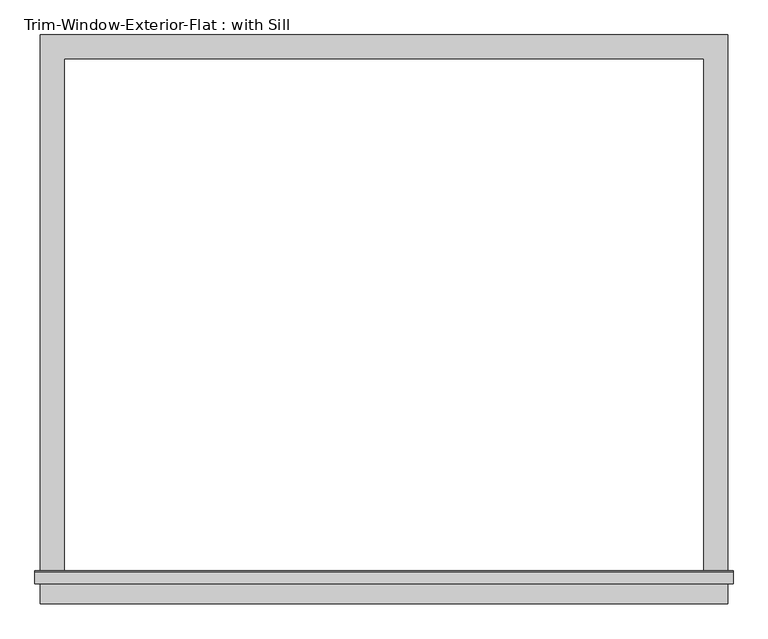
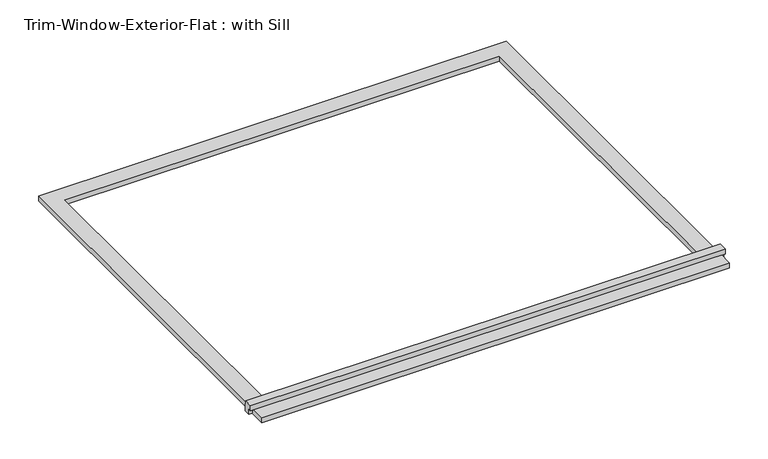
"""IFC4 building model written with IfcOpenShell, lengths in millimetres: proxy geometry, Trim-Window-Exterior-Flat : with Sill."""

from ifc_helpers import new_model, si_unit, frame, origin, origin_with_axes, place, context, project, spatial, polyline, outline, extrude, source, transform, mapped, element, save


def trim_window_exterior_flat_with_sill_7631c5ba(model_context):
    return source(origin(), model_context, "Body", "SweptSolid", [
        extrude(outline(polyline([(819.15, -1241.3823709), (819.15, -1298.5323709), (-819.15, -1298.5323709), (-819.15, -1241.3823709), (819.15, -1241.3823709)])), origin_with_axes(), (0.0, 0.0, 1.0), 19.05),
        extrude(outline(polyline([(-1250.95, 38.1), (-1221.6580645, 38.1), (-1219.2, 19.05), (-1219.2, 0.0), (-1241.3823709, 0.0), (-1241.3823709, 19.05), (-1250.95, 19.05), (-1250.95, 38.1)])), frame((-831.85, 0.0, 0.0), z_axis=(1.0, 0.0, 0.0), x_axis=(0.0, 1.0, 0.0)), (0.0, 0.0, 1.0), 1663.7),
        extrude(outline(polyline([(-819.15, 57.15), (819.15, 57.15), (819.15, -1219.2), (762.0, -1219.2), (762.0, 0.0), (-762.0, 0.0), (-762.0, -1219.2), (-819.15, -1219.2), (-819.15, 57.15)])), origin_with_axes(), (0.0, 0.0, 1.0), 19.05),
    ])


if __name__ == "__main__":
    model = new_model("IFC4")
    model_context = context("Model", 3, world=origin())
    ifc_project = project(units=[si_unit("LENGTHUNIT", "METRE", prefix="MILLI")], contexts=[model_context])
    site = spatial("IfcSite", under=ifc_project)
    building = spatial("IfcBuilding", under=site)
    placement = place(None, origin())
    trim_window_exterior_flat_with_sill_shape = trim_window_exterior_flat_with_sill_7631c5ba(model_context)
    element("IfcBuildingElementProxy", 1, Name="Trim-Window-Exterior-Flat : with Sill", ObjectType="Trim-Window-Exterior-Flat : with Sill", at=placement, inside=building, context=model_context, shape_type="MappedRepresentation", body=[
        mapped(trim_window_exterior_flat_with_sill_shape, transform((0.0, 0.0, 0.0), x_axis=(1.0, 0.0, 0.0), y_axis=(0.0, 1.0, 0.0), z_axis=(0.0, 0.0, 1.0))),
    ])
    save(model, "model.ifc")

# Revit data of these elements
# Type "Trim-Window-Exterior-Flat : with Sill"
#   Trim Width = 0' - 2 1/4"
#   Trim Thickness_Picture Frame = 0' - 1 1/4"
#   Trim Thickness_with Sill = 0' - 0 3/4"
#   Sill Thickness = 0' - 1 1/4"
#   Opening Width [instance default] = 2' - 0"
#   Opening Height [instance default] = 3' - 0"
#   Default Elevation = 4' - 0"
#   Sill = yes
#   Picture Frame = no
#   Trim Material [instance default] = none
# Element 1 (IfcBuildingElementProxy, "Trim-Window-Exterior-Flat : with Sill")
#   Opening Width = 5' - 0"
#   Opening Height = 4' - 0"
#   Trim Material = Clad - White
#   Materials on its faces: "Clad - White"
# Materials
#   "Clad - White": class "Wood", colour RGB 242 242 238, transparency 0, Cost = 0
